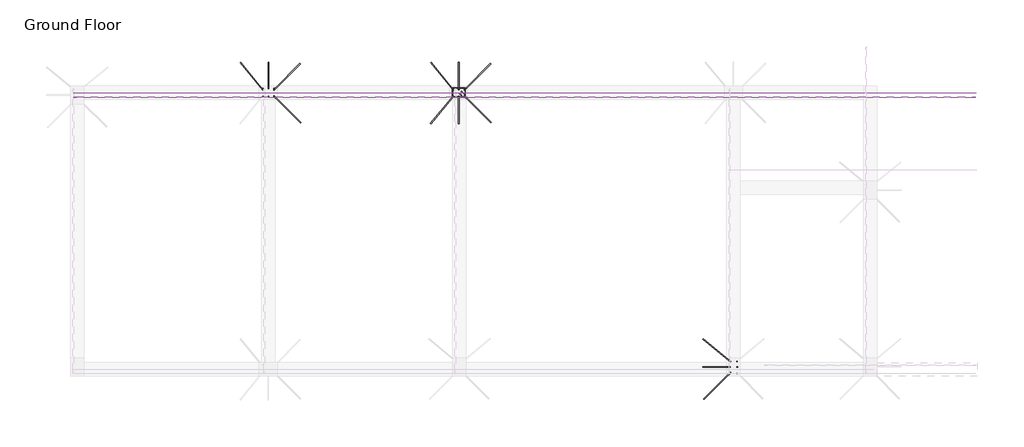
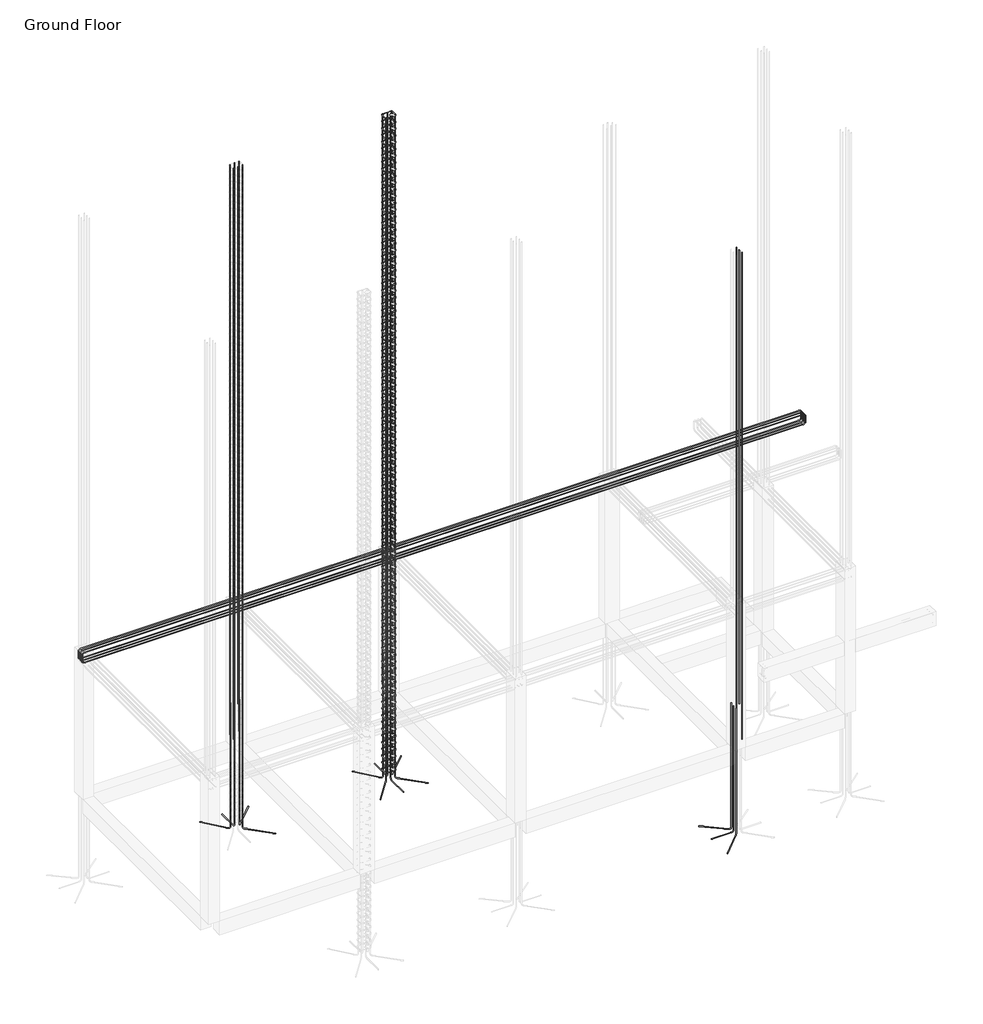
# One storey, part 4 of 5: 31 reinforcing bars.
"""IFC4 building model written with IfcOpenShell, lengths in millimetres."""

from ifc_helpers import new_model, si_unit, point, frame, origin, place, context, project, spatial, polyline, circle_curve, trimmed, segment, composite_curve, source, transform, mapped, element, save
from ifc_brep_helpers import swept_disk

model = new_model("IFC4")

# Units and contexts
model_context = context("Model", 3, world=origin())
ifc_project = project(units=[si_unit("LENGTHUNIT", "METRE", prefix="MILLI")], contexts=[model_context])

# Site, building, storey
site = spatial("IfcSite", under=ifc_project)
building = spatial("IfcBuilding", under=site)
storey = spatial("IfcBuildingStorey", under=building, Name="Ground Floor", Elevation=0.0)

# Reinforcing bars
placement = place(None, origin())
element("IfcReinforcingBar", 1, at=placement, inside=storey, context=model_context, shape_type="SolidModel", body=[
    swept_disk(composite_curve([segment(polyline([(1717.5001029, 245.6611074, 884.8983833), (1717.5001029, 245.6611074, -1868.0)]), True, "CONTINUOUS"), segment(trimmed(circle_curve(frame((1684.973191, 213.1341954, -1868.0), z_axis=(-0.7071067811865491, 0.7071067811865459, 0.0), x_axis=(32.52691189999996, 32.52691199999998, 0.0)), 46.0), [point((1717.5001029, 245.6611074, -1868.0))], [point((1684.973191, 213.1341954, -1914.0))], True, "CARTESIAN"), True, "CONTINUOUS"), segment(polyline([(1684.973191, 213.1341954, -1914.0), (1272.8436572, -198.9953384, -1914.0)]), True, "CONTINUOUS")], self_intersect=False), 6.0),
])
element("IfcReinforcingBar", 2, at=placement, inside=storey, context=model_context, shape_type="SolidModel", body=[
    swept_disk(composite_curve([segment(polyline([(1718.3160253, 432.7322479, 890.3940928), (1718.3160253, 432.7322479, -1868.0)]), True, "CONTINUOUS"), segment(trimmed(circle_curve(frame((1682.7699549, 461.9294546, -1868.0), z_axis=(0.6347218846289029, 0.7727406610067401, 0.0), x_axis=(35.54607040000019, -29.19720669999998, 0.0)), 46.0), [point((1718.3160253, 432.7322479, -1868.0))], [point((1682.7699549, 461.9294546, -1914.0))], True, "CARTESIAN"), True, "CONTINUOUS"), segment(polyline([(1682.7699549, 461.9294546, -1914.0), (1258.6023125, 810.3367522, -1914.0)]), True, "CONTINUOUS")], self_intersect=False), 6.0),
])
element("IfcReinforcingBar", 3, at=placement, inside=storey, context=model_context, shape_type="SolidModel", body=[
    swept_disk(composite_curve([segment(polyline([(1711.3882476, 339.6230123, 879.2840812), (1711.3882476, 339.6230123, -1868.0)]), True, "CONTINUOUS"), segment(trimmed(circle_curve(frame((1665.3882476, 339.6230123, -1868.0), z_axis=(0.0, 1.0, 0.0), x_axis=(46.0, 0.0, 0.0)), 46.0), [point((1711.3882476, 339.6230123, -1868.0))], [point((1665.3882476, 339.6230123, -1914.0))], True, "CARTESIAN"), True, "CONTINUOUS"), segment(polyline([(1665.3882476, 339.6230123, -1914.0), (1251.8777923, 339.6230123, -1914.0)]), True, "CONTINUOUS")], self_intersect=False), 6.0),
])
element("IfcReinforcingBar", 4, at=placement, inside=storey, context=model_context, shape_type="SolidModel", body=[
    swept_disk(composite_curve([segment(polyline([(1827.8877425, 229.5339681, 10959.9782803), (1827.8877425, 229.5339681, 171.0746196)]), True, "CONTINUOUS")], self_intersect=False), 6.0),
])
element("IfcReinforcingBar", 5, at=placement, inside=storey, context=model_context, shape_type="SolidModel", body=[
    swept_disk(composite_curve([segment(polyline([(1831.9882476, 339.6230123, 888.7528218), (1831.9882476, 339.6230123, 10945.3576223)]), True, "CONTINUOUS")], self_intersect=False), 6.0),
])
element("IfcReinforcingBar", 6, at=placement, inside=storey, context=model_context, shape_type="SolidModel", body=[
    swept_disk(composite_curve([segment(polyline([(1827.8877425, 433.132958, 10946.3939738), (1827.8877425, 433.132958, 154.6015232)]), True, "CONTINUOUS")], self_intersect=False), 6.0),
])
element("IfcReinforcingBar", 7, at=placement, inside=storey, context=model_context, shape_type="SolidModel", body=[
    swept_disk(composite_curve([segment(polyline([(-5957.3854913, 5003.5722242, 877.2694454), (-5957.3854913, 5003.5722242, -1868.0)]), True, "CONTINUOUS"), segment(trimmed(circle_curve(frame((-5924.8585793, 5036.0991362, -1868.0), z_axis=(0.7071067811865447, -0.7071067811865503, 0.0), x_axis=(-32.526911999999356, -32.526912000000266, 0.0)), 46.0), [point((-5957.3854913, 5003.5722242, -1868.0))], [point((-5924.8585793, 5036.0991362, -1914.0))], True, "CARTESIAN"), True, "CONTINUOUS"), segment(polyline([(-5924.8585793, 5036.0991362, -1914.0), (-5519.1553199, 5441.8023956, -1914.0)]), True, "CONTINUOUS")], self_intersect=False), 6.0),
])
element("IfcReinforcingBar", 8, at=placement, inside=storey, context=model_context, shape_type="SolidModel", body=[
    swept_disk(composite_curve([segment(polyline([(-5958.3393967, 4894.7453184, 884.8983833), (-5958.3393967, 4894.7453184, -1868.0)]), True, "CONTINUOUS"), segment(trimmed(circle_curve(frame((-5925.8124848, 4862.2184065, -1868.0), z_axis=(-0.7071067811865472, -0.7071067811865479, 0.0), x_axis=(-32.526911900000414, 32.526911899999504, 0.0)), 46.0), [point((-5958.3393967, 4894.7453184, -1868.0))], [point((-5925.8124848, 4862.2184065, -1914.0))], True, "CARTESIAN"), True, "CONTINUOUS"), segment(polyline([(-5925.8124848, 4862.2184065, -1914.0), (-5513.682951, 4450.0888727, -1914.0)]), True, "CONTINUOUS")], self_intersect=False), 6.0),
])
element("IfcReinforcingBar", 9, at=placement, inside=storey, context=model_context, shape_type="SolidModel", body=[
    swept_disk(composite_curve([segment(polyline([(-6145.6650805, 5002.2623878, 871.8711989), (-6145.6650805, 5002.2623878, -1868.0)]), True, "CONTINUOUS"), segment(trimmed(circle_curve(frame((-6174.8622872, 5037.8084582, -1868.0), z_axis=(0.7727406610067411, 0.6347218846289017, 0.0), x_axis=(29.197206699999697, -35.546070399999735, 0.0)), 46.0), [point((-6145.6650805, 5002.2623878, -1868.0))], [point((-6174.8622872, 5037.8084582, -1914.0))], True, "CARTESIAN"), True, "CONTINUOUS"), segment(polyline([(-6174.8622872, 5037.8084582, -1914.0), (-6521.7650416, 5460.1443982, -1914.0)]), True, "CONTINUOUS")], self_intersect=False), 6.0),
])
element("IfcReinforcingBar", 10, at=placement, inside=storey, context=model_context, shape_type="SolidModel", body=[
    swept_disk(composite_curve([segment(polyline([(-6052.3013017, 5024.2334631, 875.7528218), (-6052.3013017, 5024.2334631, -1868.0)]), True, "CONTINUOUS"), segment(trimmed(circle_curve(frame((-6052.3013017, 5070.2334631, -1868.0), z_axis=(1.0, 0.0, 0.0), x_axis=(0.0, -46.0, 0.0)), 46.0), [point((-6052.3013017, 5024.2334631, -1868.0))], [point((-6052.3013017, 5070.2334631, -1914.0))], True, "CARTESIAN"), True, "CONTINUOUS"), segment(polyline([(-6052.3013017, 5070.2334631, -1914.0), (-6052.3013017, 5466.2092764, -1914.0)]), True, "CONTINUOUS")], self_intersect=False), 6.0),
])
element("IfcReinforcingBar", 11, at=placement, inside=storey, context=model_context, shape_type="SolidModel", body=[
    swept_disk(composite_curve([segment(polyline([(-5957.2122575, 5020.132958, 12794.2305276), (-5957.2122575, 5020.132958, 171.0746196)]), True, "CONTINUOUS")], self_intersect=False), 6.0),
])
element("IfcReinforcingBar", 12, at=placement, inside=storey, context=model_context, shape_type="SolidModel", body=[
    swept_disk(composite_curve([segment(polyline([(-6052.3013017, 5024.2334631, 888.7528218), (-6052.3013017, 5024.2334631, 12792.7935546)]), True, "CONTINUOUS")], self_intersect=False), 6.0),
])
element("IfcReinforcingBar", 13, at=placement, inside=storey, context=model_context, shape_type="SolidModel", body=[
    swept_disk(composite_curve([segment(polyline([(-6145.8112474, 5020.132958, 12790.6127039), (-6145.8112474, 5020.132958, 154.6015232)]), True, "CONTINUOUS")], self_intersect=False), 6.0),
])
element("IfcReinforcingBar", 14, at=placement, inside=storey, context=model_context, shape_type="SolidModel", body=[
    swept_disk(composite_curve([segment(polyline([(-5957.2122575, 4892.7339681, 12794.2305276), (-5957.2122575, 4892.7339681, 159.2991411)]), True, "CONTINUOUS")], self_intersect=False), 6.0),
])
element("IfcReinforcingBar", 15, at=placement, inside=storey, context=model_context, shape_type="SolidModel", body=[
    swept_disk(composite_curve([segment(polyline([(-6052.3013017, 4888.6334631, 892.2840812), (-6052.3013017, 4888.6334631, 12792.7935546)]), True, "CONTINUOUS")], self_intersect=False), 6.0),
])
element("IfcReinforcingBar", 16, at=placement, inside=storey, context=model_context, shape_type="SolidModel", body=[
    swept_disk(composite_curve([segment(polyline([(-6145.8112474, 4892.7339681, 12790.6127039), (-6145.8112474, 4892.7339681, 134.6074908)]), True, "CONTINUOUS")], self_intersect=False), 6.0),
])
element("IfcReinforcingBar", 17, at=placement, inside=storey, context=model_context, shape_type="SolidModel", body=[
    swept_disk(composite_curve([segment(polyline([(-2756.9854913, 5003.5722242, 877.2694454), (-2756.9854913, 5003.5722242, -1868.0)]), True, "CONTINUOUS"), segment(trimmed(circle_curve(frame((-2724.4585793, 5036.0991362, -1868.0), z_axis=(0.7071067811865447, -0.7071067811865503, 0.0), x_axis=(-32.52691199999981, -32.526912000000266, 0.0)), 46.0), [point((-2756.9854913, 5003.5722242, -1868.0))], [point((-2724.4585793, 5036.0991362, -1914.0))], True, "CARTESIAN"), True, "CONTINUOUS"), segment(polyline([(-2724.4585793, 5036.0991362, -1914.0), (-2318.7553199, 5441.8023956, -1914.0)]), True, "CONTINUOUS")], self_intersect=False), 6.0),
])
element("IfcReinforcingBar", 18, at=placement, inside=storey, context=model_context, shape_type="SolidModel", body=[
    swept_disk(composite_curve([segment(polyline([(-2757.9393967, 4894.7453184, 884.8983833), (-2757.9393967, 4894.7453184, -1868.0)]), True, "CONTINUOUS"), segment(trimmed(circle_curve(frame((-2725.4124848, 4862.2184065, -1868.0), z_axis=(-0.7071067811865472, -0.7071067811865479, 0.0), x_axis=(-32.52691189999996, 32.526911899999504, 0.0)), 46.0), [point((-2757.9393967, 4894.7453184, -1868.0))], [point((-2725.4124848, 4862.2184065, -1914.0))], True, "CARTESIAN"), True, "CONTINUOUS"), segment(polyline([(-2725.4124848, 4862.2184065, -1914.0), (-2313.282951, 4450.0888727, -1914.0)]), True, "CONTINUOUS")], self_intersect=False), 6.0),
])
element("IfcReinforcingBar", 19, at=placement, inside=storey, context=model_context, shape_type="SolidModel", body=[
    swept_disk(composite_curve([segment(polyline([(-2945.2650805, 5002.2623878, 871.8711989), (-2945.2650805, 5002.2623878, -1868.0)]), True, "CONTINUOUS"), segment(trimmed(circle_curve(frame((-2974.4622872, 5037.8084582, -1868.0), z_axis=(0.7727406610067413, 0.6347218846289017, 0.0), x_axis=(29.19720670000015, -35.546070399999735, 0.0)), 46.0), [point((-2945.2650805, 5002.2623878, -1868.0))], [point((-2974.4622872, 5037.8084582, -1914.0))], True, "CARTESIAN"), True, "CONTINUOUS"), segment(polyline([(-2974.4622872, 5037.8084582, -1914.0), (-3321.3650416, 5460.1443982, -1914.0)]), True, "CONTINUOUS")], self_intersect=False), 6.0),
])
element("IfcReinforcingBar", 20, at=placement, inside=storey, context=model_context, shape_type="SolidModel", body=[
    swept_disk(composite_curve([segment(polyline([(-2945.0105373, 4895.5612408, 890.3940928), (-2945.0105373, 4895.5612408, -1868.0)]), True, "CONTINUOUS"), segment(trimmed(circle_curve(frame((-2974.207744, 4860.0151704, -1868.0), z_axis=(-0.772740661006739, 0.6347218846289044, 0.0), x_axis=(29.197206699999697, 35.546070399999735, 0.0)), 46.0), [point((-2945.0105373, 4895.5612408, -1868.0))], [point((-2974.207744, 4860.0151704, -1914.0))], True, "CARTESIAN"), True, "CONTINUOUS"), segment(polyline([(-2974.207744, 4860.0151704, -1914.0), (-3322.6150416, 4435.8475279, -1914.0)]), True, "CONTINUOUS")], self_intersect=False), 6.0),
])
element("IfcReinforcingBar", 21, at=placement, inside=storey, context=model_context, shape_type="SolidModel", body=[
    swept_disk(composite_curve([segment(polyline([(-2851.9013017, 5007.3834631, 875.7528218), (-2851.9013017, 5007.3834631, -1868.0)]), True, "CONTINUOUS"), segment(trimmed(circle_curve(frame((-2851.9013017, 5053.3834631, -1868.0), z_axis=(1.0, 0.0, 0.0), x_axis=(0.0, -46.0, 0.0)), 46.0), [point((-2851.9013017, 5007.3834631, -1868.0))], [point((-2851.9013017, 5053.3834631, -1914.0))], True, "CARTESIAN"), True, "CONTINUOUS"), segment(polyline([(-2851.9013017, 5053.3834631, -1914.0), (-2851.9013017, 5466.2092764, -1914.0)]), True, "CONTINUOUS")], self_intersect=False), 6.0),
])
element("IfcReinforcingBar", 22, at=placement, inside=storey, context=model_context, shape_type="SolidModel", body=[
    swept_disk(composite_curve([segment(polyline([(-2851.9013017, 4888.6334631, 879.2840812), (-2851.9013017, 4888.6334631, -1868.0)]), True, "CONTINUOUS"), segment(trimmed(circle_curve(frame((-2851.9013017, 4842.6334631, -1868.0), z_axis=(-1.0, 0.0, 0.0), x_axis=(0.0, 46.0, 0.0)), 46.0), [point((-2851.9013017, 4888.6334631, -1868.0))], [point((-2851.9013017, 4842.6334631, -1914.0))], True, "CARTESIAN"), True, "CONTINUOUS"), segment(polyline([(-2851.9013017, 4842.6334631, -1914.0), (-2851.9013017, 4429.1230078, -1914.0)]), True, "CONTINUOUS")], self_intersect=False), 6.0),
])
reinforcing_bar_shape = source(origin(), model_context, "Body", "SolidModel", [
    swept_disk(composite_curve([segment(polyline([(-2841.2771046, 4943.2576897, -1724.0), (-2783.6823152, 4885.6629003, -1724.0)]), True, "CONTINUOUS"), segment(trimmed(circle_curve(frame((-2766.7117524, 4902.6334631, -1724.0), z_axis=(0.0, 0.0, 1.0), x_axis=(-16.970562800000152, -16.970562800000152, 0.0)), 24.0), [point((-2783.6823152, 4885.6629003, -1724.0))], [point((-2742.7117524, 4902.6334631, -1724.0))], True, "CARTESIAN"), True, "CONTINUOUS"), segment(polyline([(-2742.7117524, 4902.6334631, -1724.0), (-2742.7117524, 5010.2334631, -1724.0)]), True, "CONTINUOUS"), segment(trimmed(circle_curve(frame((-2766.7117524, 5010.2334631, -1724.0), z_axis=(0.0, 0.0, 1.0), x_axis=(24.0, 0.0, 0.0)), 24.0), [point((-2742.7117524, 5010.2334631, -1724.0))], [point((-2766.7117524, 5034.2334631, -1724.0))], True, "CARTESIAN"), True, "CONTINUOUS"), segment(polyline([(-2766.7117524, 5034.2334631, -1724.0), (-2935.5117524, 5034.2334631, -1724.0)]), True, "CONTINUOUS"), segment(trimmed(circle_curve(frame((-2935.5117524, 5010.2651209, -1725.2323055), z_axis=(0.0, -0.051346062772955794, 0.9986809209340668), x_axis=(0.0, 23.968342200000734, 1.2323054999999385)), 24.0), [point((-2935.5117524, 5034.2334631, -1724.0))], [point((-2959.5117524, 5010.2651209, -1725.2323055))], True, "CARTESIAN"), True, "CONTINUOUS"), segment(polyline([(-2959.5117524, 5010.2651209, -1725.2323055), (-2959.5117524, 4902.6018052, -1730.7676945)]), True, "CONTINUOUS"), segment(trimmed(circle_curve(frame((-2935.5117524, 4902.6018052, -1730.7676945), z_axis=(0.0, -0.051346062772955794, 0.9986809209340668), x_axis=(-24.0, 0.0, 0.0)), 24.0), [point((-2959.5117524, 4902.6018052, -1730.7676945))], [point((-2935.5117524, 4878.6334631, -1732.0))], True, "CARTESIAN"), True, "CONTINUOUS"), segment(polyline([(-2935.5117524, 4878.6334631, -1732.0), (-2766.7117524, 4878.6334631, -1732.0)]), True, "CONTINUOUS"), segment(trimmed(circle_curve(frame((-2766.7117524, 4902.6334631, -1732.0), z_axis=(0.0, 0.0, 1.0), x_axis=(0.0, -24.0, 0.0)), 24.0), [point((-2766.7117524, 4878.6334631, -1732.0))], [point((-2749.7411897, 4919.6040258, -1732.0))], True, "CARTESIAN"), True, "CONTINUOUS"), segment(polyline([(-2749.7411897, 4919.6040258, -1732.0), (-2807.3359791, 4977.1988152, -1732.0)]), True, "CONTINUOUS")], self_intersect=False), 4.0),
])
element("IfcReinforcingBar", 23, at=placement, inside=storey, context=model_context, shape_type="MappedRepresentation", body=[
    mapped(reinforcing_bar_shape, transform((0.0, 0.0, 0.0), x_axis=(1.0, 0.0, 0.0), y_axis=(0.0, 1.0, 0.0), z_axis=(0.0, 0.0, 1.0))),
    mapped(reinforcing_bar_shape, transform((0.0, 0.0, 149.5904239), x_axis=(1.0, 0.0, 0.0), y_axis=(0.0, 1.0, 0.0), z_axis=(0.0, 0.0, 1.0))),
    mapped(reinforcing_bar_shape, transform((0.0, 0.0, 299.1808479), x_axis=(1.0, 0.0, 0.0), y_axis=(0.0, 1.0, 0.0), z_axis=(0.0, 0.0, 1.0))),
    mapped(reinforcing_bar_shape, transform((0.0, 0.0, 448.7712718), x_axis=(1.0, 0.0, 0.0), y_axis=(0.0, 1.0, 0.0), z_axis=(0.0, 0.0, 1.0))),
    mapped(reinforcing_bar_shape, transform((0.0, 0.0, 598.3616957), x_axis=(1.0, 0.0, 0.0), y_axis=(0.0, 1.0, 0.0), z_axis=(0.0, 0.0, 1.0))),
    mapped(reinforcing_bar_shape, transform((0.0, 0.0, 747.9521197), x_axis=(1.0, 0.0, 0.0), y_axis=(0.0, 1.0, 0.0), z_axis=(0.0, 0.0, 1.0))),
    mapped(reinforcing_bar_shape, transform((0.0, 0.0, 897.5425436), x_axis=(1.0, 0.0, 0.0), y_axis=(0.0, 1.0, 0.0), z_axis=(0.0, 0.0, 1.0))),
    mapped(reinforcing_bar_shape, transform((0.0, 0.0, 1047.1329675), x_axis=(1.0, 0.0, 0.0), y_axis=(0.0, 1.0, 0.0), z_axis=(0.0, 0.0, 1.0))),
    mapped(reinforcing_bar_shape, transform((0.0, 0.0, 1196.7233914), x_axis=(1.0, 0.0, 0.0), y_axis=(0.0, 1.0, 0.0), z_axis=(0.0, 0.0, 1.0))),
    mapped(reinforcing_bar_shape, transform((0.0, 0.0, 1346.3138154), x_axis=(1.0, 0.0, 0.0), y_axis=(0.0, 1.0, 0.0), z_axis=(0.0, 0.0, 1.0))),
    mapped(reinforcing_bar_shape, transform((0.0, 0.0, 1495.9042393), x_axis=(1.0, 0.0, 0.0), y_axis=(0.0, 1.0, 0.0), z_axis=(0.0, 0.0, 1.0))),
    mapped(reinforcing_bar_shape, transform((0.0, 0.0, 1645.4946632), x_axis=(1.0, 0.0, 0.0), y_axis=(0.0, 1.0, 0.0), z_axis=(0.0, 0.0, 1.0))),
    mapped(reinforcing_bar_shape, transform((0.0, 0.0, 1795.0850872), x_axis=(1.0, 0.0, 0.0), y_axis=(0.0, 1.0, 0.0), z_axis=(0.0, 0.0, 1.0))),
    mapped(reinforcing_bar_shape, transform((0.0, 0.0, 1944.6755111), x_axis=(1.0, 0.0, 0.0), y_axis=(0.0, 1.0, 0.0), z_axis=(0.0, 0.0, 1.0))),
    mapped(reinforcing_bar_shape, transform((0.0, 0.0, 2094.265935), x_axis=(1.0, 0.0, 0.0), y_axis=(0.0, 1.0, 0.0), z_axis=(0.0, 0.0, 1.0))),
    mapped(reinforcing_bar_shape, transform((0.0, 0.0, 2243.856359), x_axis=(1.0, 0.0, 0.0), y_axis=(0.0, 1.0, 0.0), z_axis=(0.0, 0.0, 1.0))),
    mapped(reinforcing_bar_shape, transform((0.0, 0.0, 2393.4467829), x_axis=(1.0, 0.0, 0.0), y_axis=(0.0, 1.0, 0.0), z_axis=(0.0, 0.0, 1.0))),
    mapped(reinforcing_bar_shape, transform((0.0, 0.0, 2543.0372068), x_axis=(1.0, 0.0, 0.0), y_axis=(0.0, 1.0, 0.0), z_axis=(0.0, 0.0, 1.0))),
    mapped(reinforcing_bar_shape, transform((0.0, 0.0, 2692.6276307), x_axis=(1.0, 0.0, 0.0), y_axis=(0.0, 1.0, 0.0), z_axis=(0.0, 0.0, 1.0))),
    mapped(reinforcing_bar_shape, transform((0.0, 0.0, 2842.2180547), x_axis=(1.0, 0.0, 0.0), y_axis=(0.0, 1.0, 0.0), z_axis=(0.0, 0.0, 1.0))),
    mapped(reinforcing_bar_shape, transform((0.0, 0.0, 2991.8084786), x_axis=(1.0, 0.0, 0.0), y_axis=(0.0, 1.0, 0.0), z_axis=(0.0, 0.0, 1.0))),
    mapped(reinforcing_bar_shape, transform((0.0, 0.0, 3141.3989025), x_axis=(1.0, 0.0, 0.0), y_axis=(0.0, 1.0, 0.0), z_axis=(0.0, 0.0, 1.0))),
    mapped(reinforcing_bar_shape, transform((0.0, 0.0, 3290.9893265), x_axis=(1.0, 0.0, 0.0), y_axis=(0.0, 1.0, 0.0), z_axis=(0.0, 0.0, 1.0))),
    mapped(reinforcing_bar_shape, transform((0.0, 0.0, 3440.5797504), x_axis=(1.0, 0.0, 0.0), y_axis=(0.0, 1.0, 0.0), z_axis=(0.0, 0.0, 1.0))),
    mapped(reinforcing_bar_shape, transform((0.0, 0.0, 3590.1701743), x_axis=(1.0, 0.0, 0.0), y_axis=(0.0, 1.0, 0.0), z_axis=(0.0, 0.0, 1.0))),
    mapped(reinforcing_bar_shape, transform((0.0, 0.0, 3739.7605983), x_axis=(1.0, 0.0, 0.0), y_axis=(0.0, 1.0, 0.0), z_axis=(0.0, 0.0, 1.0))),
    mapped(reinforcing_bar_shape, transform((0.0, 0.0, 3889.3510222), x_axis=(1.0, 0.0, 0.0), y_axis=(0.0, 1.0, 0.0), z_axis=(0.0, 0.0, 1.0))),
    mapped(reinforcing_bar_shape, transform((0.0, 0.0, 4038.9414461), x_axis=(1.0, 0.0, 0.0), y_axis=(0.0, 1.0, 0.0), z_axis=(0.0, 0.0, 1.0))),
    mapped(reinforcing_bar_shape, transform((0.0, 0.0, 4188.53187), x_axis=(1.0, 0.0, 0.0), y_axis=(0.0, 1.0, 0.0), z_axis=(0.0, 0.0, 1.0))),
    mapped(reinforcing_bar_shape, transform((0.0, 0.0, 4338.122294), x_axis=(1.0, 0.0, 0.0), y_axis=(0.0, 1.0, 0.0), z_axis=(0.0, 0.0, 1.0))),
    mapped(reinforcing_bar_shape, transform((0.0, 0.0, 4487.7127179), x_axis=(1.0, 0.0, 0.0), y_axis=(0.0, 1.0, 0.0), z_axis=(0.0, 0.0, 1.0))),
    mapped(reinforcing_bar_shape, transform((0.0, 0.0, 4637.3031418), x_axis=(1.0, 0.0, 0.0), y_axis=(0.0, 1.0, 0.0), z_axis=(0.0, 0.0, 1.0))),
    mapped(reinforcing_bar_shape, transform((0.0, 0.0, 4786.8935658), x_axis=(1.0, 0.0, 0.0), y_axis=(0.0, 1.0, 0.0), z_axis=(0.0, 0.0, 1.0))),
    mapped(reinforcing_bar_shape, transform((0.0, 0.0, 4936.4839897), x_axis=(1.0, 0.0, 0.0), y_axis=(0.0, 1.0, 0.0), z_axis=(0.0, 0.0, 1.0))),
    mapped(reinforcing_bar_shape, transform((0.0, 0.0, 5086.0744136), x_axis=(1.0, 0.0, 0.0), y_axis=(0.0, 1.0, 0.0), z_axis=(0.0, 0.0, 1.0))),
    mapped(reinforcing_bar_shape, transform((0.0, 0.0, 5235.6648376), x_axis=(1.0, 0.0, 0.0), y_axis=(0.0, 1.0, 0.0), z_axis=(0.0, 0.0, 1.0))),
    mapped(reinforcing_bar_shape, transform((0.0, 0.0, 5385.2552615), x_axis=(1.0, 0.0, 0.0), y_axis=(0.0, 1.0, 0.0), z_axis=(0.0, 0.0, 1.0))),
    mapped(reinforcing_bar_shape, transform((0.0, 0.0, 5534.8456854), x_axis=(1.0, 0.0, 0.0), y_axis=(0.0, 1.0, 0.0), z_axis=(0.0, 0.0, 1.0))),
    mapped(reinforcing_bar_shape, transform((0.0, 0.0, 5684.4361094), x_axis=(1.0, 0.0, 0.0), y_axis=(0.0, 1.0, 0.0), z_axis=(0.0, 0.0, 1.0))),
    mapped(reinforcing_bar_shape, transform((0.0, 0.0, 5834.0265333), x_axis=(1.0, 0.0, 0.0), y_axis=(0.0, 1.0, 0.0), z_axis=(0.0, 0.0, 1.0))),
    mapped(reinforcing_bar_shape, transform((0.0, 0.0, 5983.6169572), x_axis=(1.0, 0.0, 0.0), y_axis=(0.0, 1.0, 0.0), z_axis=(0.0, 0.0, 1.0))),
    mapped(reinforcing_bar_shape, transform((0.0, 0.0, 6133.2073811), x_axis=(1.0, 0.0, 0.0), y_axis=(0.0, 1.0, 0.0), z_axis=(0.0, 0.0, 1.0))),
    mapped(reinforcing_bar_shape, transform((0.0, 0.0, 6282.7978051), x_axis=(1.0, 0.0, 0.0), y_axis=(0.0, 1.0, 0.0), z_axis=(0.0, 0.0, 1.0))),
    mapped(reinforcing_bar_shape, transform((0.0, 0.0, 6432.388229), x_axis=(1.0, 0.0, 0.0), y_axis=(0.0, 1.0, 0.0), z_axis=(0.0, 0.0, 1.0))),
    mapped(reinforcing_bar_shape, transform((0.0, 0.0, 6581.9786529), x_axis=(1.0, 0.0, 0.0), y_axis=(0.0, 1.0, 0.0), z_axis=(0.0, 0.0, 1.0))),
    mapped(reinforcing_bar_shape, transform((0.0, 0.0, 6731.5690769), x_axis=(1.0, 0.0, 0.0), y_axis=(0.0, 1.0, 0.0), z_axis=(0.0, 0.0, 1.0))),
    mapped(reinforcing_bar_shape, transform((0.0, 0.0, 6881.1595008), x_axis=(1.0, 0.0, 0.0), y_axis=(0.0, 1.0, 0.0), z_axis=(0.0, 0.0, 1.0))),
    mapped(reinforcing_bar_shape, transform((0.0, 0.0, 7030.7499247), x_axis=(1.0, 0.0, 0.0), y_axis=(0.0, 1.0, 0.0), z_axis=(0.0, 0.0, 1.0))),
    mapped(reinforcing_bar_shape, transform((0.0, 0.0, 7180.3403487), x_axis=(1.0, 0.0, 0.0), y_axis=(0.0, 1.0, 0.0), z_axis=(0.0, 0.0, 1.0))),
    mapped(reinforcing_bar_shape, transform((0.0, 0.0, 7329.9307726), x_axis=(1.0, 0.0, 0.0), y_axis=(0.0, 1.0, 0.0), z_axis=(0.0, 0.0, 1.0))),
    mapped(reinforcing_bar_shape, transform((0.0, 0.0, 7479.5211965), x_axis=(1.0, 0.0, 0.0), y_axis=(0.0, 1.0, 0.0), z_axis=(0.0, 0.0, 1.0))),
    mapped(reinforcing_bar_shape, transform((0.0, 0.0, 7629.1116204), x_axis=(1.0, 0.0, 0.0), y_axis=(0.0, 1.0, 0.0), z_axis=(0.0, 0.0, 1.0))),
    mapped(reinforcing_bar_shape, transform((0.0, 0.0, 7778.7020444), x_axis=(1.0, 0.0, 0.0), y_axis=(0.0, 1.0, 0.0), z_axis=(0.0, 0.0, 1.0))),
    mapped(reinforcing_bar_shape, transform((0.0, 0.0, 7928.2924683), x_axis=(1.0, 0.0, 0.0), y_axis=(0.0, 1.0, 0.0), z_axis=(0.0, 0.0, 1.0))),
    mapped(reinforcing_bar_shape, transform((0.0, 0.0, 8077.8828922), x_axis=(1.0, 0.0, 0.0), y_axis=(0.0, 1.0, 0.0), z_axis=(0.0, 0.0, 1.0))),
    mapped(reinforcing_bar_shape, transform((0.0, 0.0, 8227.4733162), x_axis=(1.0, 0.0, 0.0), y_axis=(0.0, 1.0, 0.0), z_axis=(0.0, 0.0, 1.0))),
    mapped(reinforcing_bar_shape, transform((0.0, 0.0, 8377.0637401), x_axis=(1.0, 0.0, 0.0), y_axis=(0.0, 1.0, 0.0), z_axis=(0.0, 0.0, 1.0))),
    mapped(reinforcing_bar_shape, transform((0.0, 0.0, 8526.654164), x_axis=(1.0, 0.0, 0.0), y_axis=(0.0, 1.0, 0.0), z_axis=(0.0, 0.0, 1.0))),
    mapped(reinforcing_bar_shape, transform((0.0, 0.0, 8676.244588), x_axis=(1.0, 0.0, 0.0), y_axis=(0.0, 1.0, 0.0), z_axis=(0.0, 0.0, 1.0))),
    mapped(reinforcing_bar_shape, transform((0.0, 0.0, 8825.8350119), x_axis=(1.0, 0.0, 0.0), y_axis=(0.0, 1.0, 0.0), z_axis=(0.0, 0.0, 1.0))),
    mapped(reinforcing_bar_shape, transform((0.0, 0.0, 8975.4254358), x_axis=(1.0, 0.0, 0.0), y_axis=(0.0, 1.0, 0.0), z_axis=(0.0, 0.0, 1.0))),
    mapped(reinforcing_bar_shape, transform((0.0, 0.0, 9125.0158597), x_axis=(1.0, 0.0, 0.0), y_axis=(0.0, 1.0, 0.0), z_axis=(0.0, 0.0, 1.0))),
    mapped(reinforcing_bar_shape, transform((0.0, 0.0, 9274.6062837), x_axis=(1.0, 0.0, 0.0), y_axis=(0.0, 1.0, 0.0), z_axis=(0.0, 0.0, 1.0))),
    mapped(reinforcing_bar_shape, transform((0.0, 0.0, 9424.1967076), x_axis=(1.0, 0.0, 0.0), y_axis=(0.0, 1.0, 0.0), z_axis=(0.0, 0.0, 1.0))),
    mapped(reinforcing_bar_shape, transform((0.0, 0.0, 9573.7871315), x_axis=(1.0, 0.0, 0.0), y_axis=(0.0, 1.0, 0.0), z_axis=(0.0, 0.0, 1.0))),
    mapped(reinforcing_bar_shape, transform((0.0, 0.0, 9723.3775555), x_axis=(1.0, 0.0, 0.0), y_axis=(0.0, 1.0, 0.0), z_axis=(0.0, 0.0, 1.0))),
    mapped(reinforcing_bar_shape, transform((0.0, 0.0, 9872.9679794), x_axis=(1.0, 0.0, 0.0), y_axis=(0.0, 1.0, 0.0), z_axis=(0.0, 0.0, 1.0))),
    mapped(reinforcing_bar_shape, transform((0.0, 0.0, 10022.5584033), x_axis=(1.0, 0.0, 0.0), y_axis=(0.0, 1.0, 0.0), z_axis=(0.0, 0.0, 1.0))),
    mapped(reinforcing_bar_shape, transform((0.0, 0.0, 10172.1488273), x_axis=(1.0, 0.0, 0.0), y_axis=(0.0, 1.0, 0.0), z_axis=(0.0, 0.0, 1.0))),
    mapped(reinforcing_bar_shape, transform((0.0, 0.0, 10321.7392512), x_axis=(1.0, 0.0, 0.0), y_axis=(0.0, 1.0, 0.0), z_axis=(0.0, 0.0, 1.0))),
    mapped(reinforcing_bar_shape, transform((0.0, 0.0, 10471.3296751), x_axis=(1.0, 0.0, 0.0), y_axis=(0.0, 1.0, 0.0), z_axis=(0.0, 0.0, 1.0))),
    mapped(reinforcing_bar_shape, transform((0.0, 0.0, 10620.9200991), x_axis=(1.0, 0.0, 0.0), y_axis=(0.0, 1.0, 0.0), z_axis=(0.0, 0.0, 1.0))),
    mapped(reinforcing_bar_shape, transform((0.0, 0.0, 10770.510523), x_axis=(1.0, 0.0, 0.0), y_axis=(0.0, 1.0, 0.0), z_axis=(0.0, 0.0, 1.0))),
    mapped(reinforcing_bar_shape, transform((0.0, 0.0, 10920.1009469), x_axis=(1.0, 0.0, 0.0), y_axis=(0.0, 1.0, 0.0), z_axis=(0.0, 0.0, 1.0))),
    mapped(reinforcing_bar_shape, transform((0.0, 0.0, 11069.6913708), x_axis=(1.0, 0.0, 0.0), y_axis=(0.0, 1.0, 0.0), z_axis=(0.0, 0.0, 1.0))),
    mapped(reinforcing_bar_shape, transform((0.0, 0.0, 11219.2817948), x_axis=(1.0, 0.0, 0.0), y_axis=(0.0, 1.0, 0.0), z_axis=(0.0, 0.0, 1.0))),
    mapped(reinforcing_bar_shape, transform((0.0, 0.0, 11368.8722187), x_axis=(1.0, 0.0, 0.0), y_axis=(0.0, 1.0, 0.0), z_axis=(0.0, 0.0, 1.0))),
    mapped(reinforcing_bar_shape, transform((0.0, 0.0, 11518.4626426), x_axis=(1.0, 0.0, 0.0), y_axis=(0.0, 1.0, 0.0), z_axis=(0.0, 0.0, 1.0))),
    mapped(reinforcing_bar_shape, transform((0.0, 0.0, 11668.0530666), x_axis=(1.0, 0.0, 0.0), y_axis=(0.0, 1.0, 0.0), z_axis=(0.0, 0.0, 1.0))),
    mapped(reinforcing_bar_shape, transform((0.0, 0.0, 11817.6434905), x_axis=(1.0, 0.0, 0.0), y_axis=(0.0, 1.0, 0.0), z_axis=(0.0, 0.0, 1.0))),
    mapped(reinforcing_bar_shape, transform((0.0, 0.0, 11967.2339144), x_axis=(1.0, 0.0, 0.0), y_axis=(0.0, 1.0, 0.0), z_axis=(0.0, 0.0, 1.0))),
    mapped(reinforcing_bar_shape, transform((0.0, 0.0, 12116.8243384), x_axis=(1.0, 0.0, 0.0), y_axis=(0.0, 1.0, 0.0), z_axis=(0.0, 0.0, 1.0))),
    mapped(reinforcing_bar_shape, transform((0.0, 0.0, 12266.4147623), x_axis=(1.0, 0.0, 0.0), y_axis=(0.0, 1.0, 0.0), z_axis=(0.0, 0.0, 1.0))),
    mapped(reinforcing_bar_shape, transform((0.0, 0.0, 12416.0051862), x_axis=(1.0, 0.0, 0.0), y_axis=(0.0, 1.0, 0.0), z_axis=(0.0, 0.0, 1.0))),
    mapped(reinforcing_bar_shape, transform((0.0, 0.0, 12565.5956101), x_axis=(1.0, 0.0, 0.0), y_axis=(0.0, 1.0, 0.0), z_axis=(0.0, 0.0, 1.0))),
    mapped(reinforcing_bar_shape, transform((0.0, 0.0, 12715.1860341), x_axis=(1.0, 0.0, 0.0), y_axis=(0.0, 1.0, 0.0), z_axis=(0.0, 0.0, 1.0))),
    mapped(reinforcing_bar_shape, transform((0.0, 0.0, 12864.776458), x_axis=(1.0, 0.0, 0.0), y_axis=(0.0, 1.0, 0.0), z_axis=(0.0, 0.0, 1.0))),
    mapped(reinforcing_bar_shape, transform((0.0, 0.0, 13014.3668819), x_axis=(1.0, 0.0, 0.0), y_axis=(0.0, 1.0, 0.0), z_axis=(0.0, 0.0, 1.0))),
    mapped(reinforcing_bar_shape, transform((0.0, 0.0, 13163.9573059), x_axis=(1.0, 0.0, 0.0), y_axis=(0.0, 1.0, 0.0), z_axis=(0.0, 0.0, 1.0))),
    mapped(reinforcing_bar_shape, transform((0.0, 0.0, 13313.5477298), x_axis=(1.0, 0.0, 0.0), y_axis=(0.0, 1.0, 0.0), z_axis=(0.0, 0.0, 1.0))),
    mapped(reinforcing_bar_shape, transform((0.0, 0.0, 13463.1381537), x_axis=(1.0, 0.0, 0.0), y_axis=(0.0, 1.0, 0.0), z_axis=(0.0, 0.0, 1.0))),
    mapped(reinforcing_bar_shape, transform((0.0, 0.0, 13612.7285777), x_axis=(1.0, 0.0, 0.0), y_axis=(0.0, 1.0, 0.0), z_axis=(0.0, 0.0, 1.0))),
    mapped(reinforcing_bar_shape, transform((0.0, 0.0, 13762.3190016), x_axis=(1.0, 0.0, 0.0), y_axis=(0.0, 1.0, 0.0), z_axis=(0.0, 0.0, 1.0))),
    mapped(reinforcing_bar_shape, transform((0.0, 0.0, 13911.9094255), x_axis=(1.0, 0.0, 0.0), y_axis=(0.0, 1.0, 0.0), z_axis=(0.0, 0.0, 1.0))),
    mapped(reinforcing_bar_shape, transform((0.0, 0.0, 14061.4998494), x_axis=(1.0, 0.0, 0.0), y_axis=(0.0, 1.0, 0.0), z_axis=(0.0, 0.0, 1.0))),
    mapped(reinforcing_bar_shape, transform((0.0, 0.0, 14211.0902734), x_axis=(1.0, 0.0, 0.0), y_axis=(0.0, 1.0, 0.0), z_axis=(0.0, 0.0, 1.0))),
    mapped(reinforcing_bar_shape, transform((0.0, 0.0, 14360.6806973), x_axis=(1.0, 0.0, 0.0), y_axis=(0.0, 1.0, 0.0), z_axis=(0.0, 0.0, 1.0))),
    mapped(reinforcing_bar_shape, transform((0.0, 0.0, 14510.2711212), x_axis=(1.0, 0.0, 0.0), y_axis=(0.0, 1.0, 0.0), z_axis=(0.0, 0.0, 1.0))),
])
element("IfcReinforcingBar", 24, at=placement, inside=storey, context=model_context, shape_type="SolidModel", body=[
    swept_disk(composite_curve([segment(polyline([(-2756.8122575, 5020.132958, 12794.2305276), (-2756.8122575, 5020.132958, 171.0746196)]), True, "CONTINUOUS")], self_intersect=False), 6.0),
])
element("IfcReinforcingBar", 25, at=placement, inside=storey, context=model_context, shape_type="SolidModel", body=[
    swept_disk(composite_curve([segment(polyline([(-2851.9013017, 5007.3834631, 888.7528218), (-2851.9013017, 5007.3834631, 12792.7935546)]), True, "CONTINUOUS")], self_intersect=False), 6.0),
])
element("IfcReinforcingBar", 26, at=placement, inside=storey, context=model_context, shape_type="SolidModel", body=[
    swept_disk(composite_curve([segment(polyline([(-2945.4112474, 5020.132958, 12790.6127039), (-2945.4112474, 5020.132958, 154.6015232)]), True, "CONTINUOUS")], self_intersect=False), 6.0),
])
element("IfcReinforcingBar", 27, at=placement, inside=storey, context=model_context, shape_type="SolidModel", body=[
    swept_disk(composite_curve([segment(polyline([(-2756.8122575, 4892.7339681, 12794.2305276), (-2756.8122575, 4892.7339681, 159.2991411)]), True, "CONTINUOUS")], self_intersect=False), 6.0),
])
element("IfcReinforcingBar", 28, at=placement, inside=storey, context=model_context, shape_type="SolidModel", body=[
    swept_disk(composite_curve([segment(polyline([(-2851.9013017, 4888.6334631, 892.2840812), (-2851.9013017, 4888.6334631, 12792.7935546)]), True, "CONTINUOUS")], self_intersect=False), 6.0),
])
element("IfcReinforcingBar", 29, at=placement, inside=storey, context=model_context, shape_type="SolidModel", body=[
    swept_disk(composite_curve([segment(polyline([(-2945.4112474, 4892.7339681, 12790.6127039), (-2945.4112474, 4892.7339681, 134.6074908)]), True, "CONTINUOUS")], self_intersect=False), 6.0),
])
reinforcing_bar_2_shape = source(origin(), model_context, "Body", "SolidModel", [
    swept_disk(composite_curve([segment(polyline([(-9325.7296265, 4877.7339681, 2963.2994949), (-9325.7296265, 4877.7339681, 3111.2994949)]), True, "CONTINUOUS"), segment(trimmed(circle_curve(frame((-9279.7296265, 4877.7339681, 3111.2994949), z_axis=(0.0, 1.0, 0.0), x_axis=(-46.0, 0.0, 0.0)), 46.0), [point((-9325.7296265, 4877.7339681, 3111.2994949))], [point((-9279.7296265, 4877.7339681, 3157.2994949))], True, "CARTESIAN"), True, "CONTINUOUS"), segment(polyline([(-9279.7296265, 4877.7339681, 3157.2994949), (5794.6882476, 4877.7339681, 3157.2994949)]), True, "CONTINUOUS"), segment(trimmed(circle_curve(frame((5794.6882476, 4877.7339681, 3111.2994949), z_axis=(0.0, 1.0, 0.0), x_axis=(0.0, 0.0, 46.0)), 46.0), [point((5794.6882476, 4877.7339681, 3157.2994949))], [point((5840.6882476, 4877.7339681, 3111.2994949))], True, "CARTESIAN"), True, "CONTINUOUS"), segment(polyline([(5840.6882476, 4877.7339681, 3111.2994949), (5840.6882476, 4877.7339681, 2963.2994949)]), True, "CONTINUOUS")], self_intersect=False), 6.0),
])
element("IfcReinforcingBar", 30, at=placement, inside=storey, context=model_context, shape_type="MappedRepresentation", body=[
    mapped(reinforcing_bar_2_shape, transform((0.0, 0.0, 0.0), x_axis=(1.0, 0.0, 0.0), y_axis=(0.0, 1.0, 0.0), z_axis=(0.0, 0.0, 1.0))),
    mapped(reinforcing_bar_2_shape, transform((0.0, 71.1994949, 0.0), x_axis=(1.0, 0.0, 0.0), y_axis=(0.0, 1.0, 0.0), z_axis=(0.0, 0.0, 1.0))),
    mapped(reinforcing_bar_2_shape, transform((0.0, 142.3989899, 0.0), x_axis=(1.0, 0.0, 0.0), y_axis=(0.0, 1.0, 0.0), z_axis=(0.0, 0.0, 1.0))),
])
reinforcing_bar_3_shape = source(origin(), model_context, "Body", "SolidModel", [
    swept_disk(composite_curve([segment(polyline([(-9326.1203644, 4877.7339681, 3132.7005051), (-9326.1203644, 4877.7339681, 2984.7005051)]), True, "CONTINUOUS"), segment(trimmed(circle_curve(frame((-9280.1203644, 4877.7339681, 2984.7005051), z_axis=(0.0, -1.0, 0.0), x_axis=(-46.0, 0.0, 0.0)), 46.0), [point((-9326.1203644, 4877.7339681, 2984.7005051))], [point((-9280.1203644, 4877.7339681, 2938.7005051))], True, "CARTESIAN"), True, "CONTINUOUS"), segment(polyline([(-9280.1203644, 4877.7339681, 2938.7005051), (5783.0951301, 4877.7339681, 2938.7005051)]), True, "CONTINUOUS"), segment(trimmed(circle_curve(frame((5783.0951301, 4877.7339681, 2984.7005051), z_axis=(0.0, -1.0, 0.0), x_axis=(0.0, 0.0, -46.0)), 46.0), [point((5783.0951301, 4877.7339681, 2938.7005051))], [point((5829.0951301, 4877.7339681, 2984.7005051))], True, "CARTESIAN"), True, "CONTINUOUS"), segment(polyline([(5829.0951301, 4877.7339681, 2984.7005051), (5829.0951301, 4877.7339681, 3132.7005051)]), True, "CONTINUOUS")], self_intersect=False), 6.0),
])
element("IfcReinforcingBar", 31, at=placement, inside=storey, context=model_context, shape_type="MappedRepresentation", body=[
    mapped(reinforcing_bar_3_shape, transform((0.0, 0.0, 0.0), x_axis=(1.0, 0.0, 0.0), y_axis=(0.0, 1.0, 0.0), z_axis=(0.0, 0.0, 1.0))),
    mapped(reinforcing_bar_3_shape, transform((0.0, 71.1994949, 0.0), x_axis=(1.0, 0.0, 0.0), y_axis=(0.0, 1.0, 0.0), z_axis=(0.0, 0.0, 1.0))),
    mapped(reinforcing_bar_3_shape, transform((0.0, 142.3989899, 0.0), x_axis=(1.0, 0.0, 0.0), y_axis=(0.0, 1.0, 0.0), z_axis=(0.0, 0.0, 1.0))),
])

save(model, "model.ifc")

# Revit data of these elements
# Elements 1, 2, 3, 4, 5, 6, 7, 8, 9, 10, 11, 12, 13, 14, 15, 16, 17, 18, 19, 20, 21, 22, 23, 24, 25, 26, 27, 28, 29, 30, 31 (IfcReinforcingBar)
#   Phase Created = New Construction
